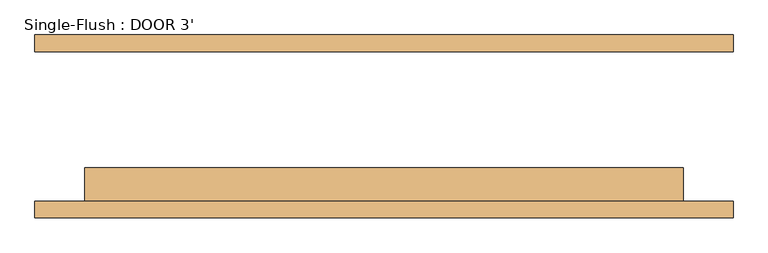
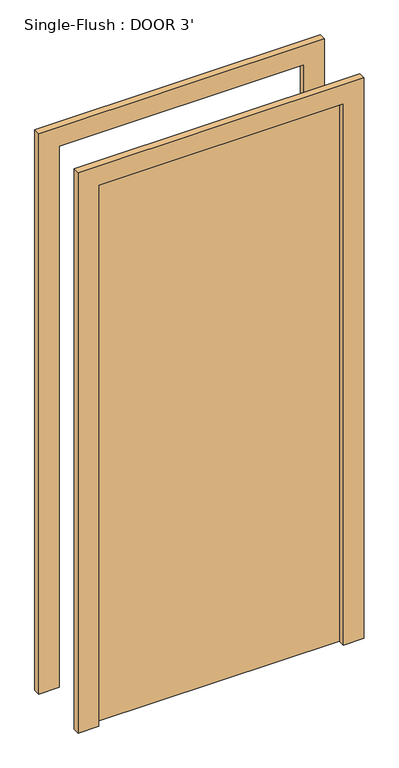
"""IFC4 building model written with IfcOpenShell, lengths in millimetres: door geometry, Single-Flush : DOOR 3'."""

from ifc_helpers import new_model, si_unit, frame, origin, origin_with_axes, place, context, project, spatial, polyline, outline, extrude, source, transform, mapped, element, save


def single_flush_door_3_a90ba1ad(model_context):
    return source(origin(), model_context, "Body", "SweptSolid", [
        extrude(outline(polyline([(2209.8, -533.4), (0.0, -533.4), (0.0, -457.2), (2133.6, -457.2), (2133.6, 457.2), (0.0, 457.2), (0.0, 533.4), (2209.8, 533.4), (2209.8, -533.4)])), frame((0.0, -139.7, 0.0), z_axis=(0.0, 1.0, 0.0), x_axis=(0.0, 0.0, 1.0)), (0.0, 0.0, 1.0), 25.4),
        extrude(outline(polyline([(2209.8, 533.4), (2209.8, -533.4), (0.0, -533.4), (0.0, -457.2), (2133.6, -457.2), (2133.6, 457.2), (0.0, 457.2), (0.0, 533.4), (2209.8, 533.4)])), frame((0.0, 114.3, 0.0), z_axis=(0.0, 1.0, 0.0), x_axis=(0.0, 0.0, 1.0)), (0.0, 0.0, 1.0), 25.4),
        extrude(outline(polyline([(457.2, -63.5), (457.2, -114.3), (-457.2, -114.3), (-457.2, -63.5), (457.2, -63.5)])), origin_with_axes(), (0.0, 0.0, 1.0), 2133.6),
    ])


if __name__ == "__main__":
    model = new_model("IFC4")
    model_context = context("Model", 3, world=origin())
    ifc_project = project(units=[si_unit("LENGTHUNIT", "METRE", prefix="MILLI")], contexts=[model_context])
    site = spatial("IfcSite", under=ifc_project)
    building = spatial("IfcBuilding", under=site)
    placement = place(None, origin())
    single_flush_door_3_shape = single_flush_door_3_a90ba1ad(model_context)
    element("IfcDoor", 1, ObjectType="Single-Flush : DOOR 3'", at=placement, inside=building, context=model_context, shape_type="MappedRepresentation", body=[
        mapped(single_flush_door_3_shape, transform((0.0, 0.0, 0.0), x_axis=(1.0, 0.0, 0.0), y_axis=(0.0, 1.0, 0.0), z_axis=(0.0, 0.0, 1.0))),
    ])
    save(model, "model.ifc")

# Revit data of these elements
# Type "Single-Flush : DOOR 3'"
#   Type Mark = "9"
#   Construction Type Id = "MDOOR"
#   Assembly Code = "C1020"
#   Analytic Construction = "Metal"
#   Thickness = 0' - 2"
#   Heat Transfer Coefficient (U) = 0.651978 BTU/(h·ft²·°F)
#   Height = 7' - 0"
#   Trim Projection Ext = 0' - 1"
#   Trim Projection Int = 0' - 1"
#   Trim Width = 0' - 3"
#   Width = 3' - 0"
#   Define Thermal Properties by = 1
#   Door Material = Door - Panel
#   Frame Material = Door - Frame
#   Visual Light Transmittance = 0
#   Solar Heat Gain Coefficient = 0
#   Function = (empty or 0)
#   Wall Closure = (empty or 0)
# Element 1 (IfcDoor, "Single-Flush : DOOR 3'")
#   Materials on its faces: "Door - Frame", "Door - Panel"
# Materials
#   "Door - Panel": class "Wood", colour RGB 210 159 95, transparency 0, Cost = 0
#   "Door - Frame": colour RGB 118 70 51, transparency 0, Cost = 0
